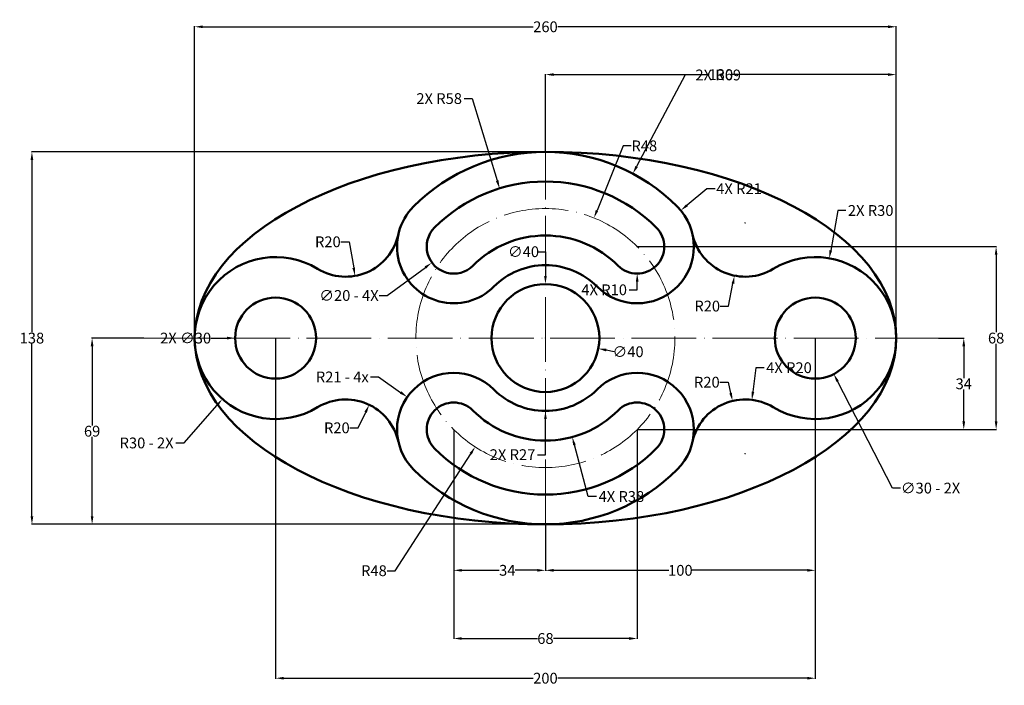
# Model space of a CAD drawing. Units: inches. Extents: x 400 to 765, y 244 to 491.
import ezdxf

# ---------------------------------------------------------------- set-up
doc = ezdxf.new("R2010")
doc.units = ezdxf.units.IN
doc.header["$MEASUREMENT"] = 0
doc.linetypes.add('ACAD_ISO04W100', pattern=[30, 24, -3, 0, -3])
for name, color, linetype, lineweight in [('M-CNTR', 4, 'ACAD_ISO04W100', 18), ('M-CONS', 8, 'Continuous', 13), ('M-DIMS', 7, 'Continuous', 25), ('M-OUTL', 7, 'Continuous', 50)]:
    doc.layers.add(name, color=color, linetype=linetype, lineweight=lineweight)
doc.styles.get("Standard").update_dxf_attribs({"font": 'arial.ttf'})
doc.dimstyles.get("Standard").update_dxf_attribs({"dimtxt": 4, "dimasz": 3, "dimexe": 0.18, "dimexo": 0.0625, "dimgap": 0.09, "dimtad": 0, "dimtih": 1, "dimtoh": 1, "dimdec": 0, "dimzin": 0, "dimdsep": 46, "dimtxsty": 'Standard', "dimcen": 0.09, "dimclrd": 1, "dimclre": 1, "dimadec": 0, "dimazin": 0, "dimtfac": 1, "dimtdec": 0, "dimtofl": 0, "dimtmove": 0, "dimatfit": 3, "dimfxl": 1, "dimtolj": 1, "dimtzin": 0, "dimarcsym": 0})

# ---------------------------------------------------------------- blocks, each defined once
blk = doc.blocks.new('*D1')
at = {"layer": 'Defpoints', "color": 0, "transparency": 16777216}
for p in [(725.07, 488.39), (465.07, 373.06), (725.07, 373.06)]:
    blk.add_point(p, dxfattribs=at)
at = {"layer": 'M-DIMS', "color": 0, "lineweight": -2, "transparency": 16777216}
for p, q in [((465.07, 373.12), (465.07, 488.57)), ((468.07, 488.39), (590.53, 488.39)), ((722.07, 488.39), (599.6, 488.39)), ((725.07, 373.12), (725.07, 488.57))]:
    blk.add_line(p, q, dxfattribs=at)
at = {"layer": 'M-DIMS', "color": 0, "transparency": 16777216}
for points in [[(468.07, 488.89), (468.07, 487.89), (465.07, 488.39)], [(722.07, 488.89), (722.07, 487.89), (725.07, 488.39)]]:
    blk.add_solid(points, dxfattribs=at)
at = {"layer": 'M-DIMS', "color": 0, "transparency": 16777216, "insert": (595.07, 488.39), "char_height": 4, "attachment_point": 5}
blk.add_mtext('\\A1;260', dxfattribs=at)
blk = doc.blocks.new('*D2')
at = {"layer": 'Defpoints', "color": 0, "transparency": 16777216}
for p in [(725.07, 470.68), (595.07, 442.06), (725.07, 373.06)]:
    blk.add_point(p, dxfattribs=at)
at = {"layer": 'M-DIMS', "color": 0, "lineweight": -2, "transparency": 16777216}
for p, q in [((595.07, 442.12), (595.07, 470.86)), ((725.07, 373.12), (725.07, 470.86)), ((598.07, 470.68), (655.75, 470.68)), ((722.07, 470.68), (664.38, 470.68))]:
    blk.add_line(p, q, dxfattribs=at)
at = {"layer": 'M-DIMS', "color": 0, "transparency": 16777216}
for points in [[(598.07, 471.18), (598.07, 470.18), (595.07, 470.68)], [(722.07, 471.18), (722.07, 470.18), (725.07, 470.68)]]:
    blk.add_solid(points, dxfattribs=at)
at = {"layer": 'M-DIMS', "color": 0, "transparency": 16777216, "insert": (660.07, 470.68), "char_height": 4, "attachment_point": 5}
blk.add_mtext('\\A1;130', dxfattribs=at)
blk = doc.blocks.new('*D3')
at = {"layer": 'Defpoints', "color": 0, "transparency": 16777216}
for p in [(595.07, 442.06), (404.77, 304.06), (595.07, 304.06)]:
    blk.add_point(p, dxfattribs=at)
at = {"layer": 'M-DIMS', "color": 0, "lineweight": -2, "transparency": 16777216}
for p, q in [((595.01, 442.06), (404.59, 442.06)), ((404.77, 439.06), (404.77, 375.19)), ((404.77, 307.06), (404.77, 370.93)), ((595.01, 304.06), (404.59, 304.06))]:
    blk.add_line(p, q, dxfattribs=at)
at = {"layer": 'M-DIMS', "color": 0, "transparency": 16777216}
for points in [[(404.27, 439.06), (405.27, 439.06), (404.77, 442.06)], [(404.27, 307.06), (405.27, 307.06), (404.77, 304.06)]]:
    blk.add_solid(points, dxfattribs=at)
at = {"layer": 'M-DIMS', "color": 0, "transparency": 16777216, "insert": (404.77, 373.06), "char_height": 4, "attachment_point": 5}
blk.add_mtext('\\A1;138', dxfattribs=at)
blk = doc.blocks.new('*D4')
at = {"layer": 'Defpoints', "color": 0, "transparency": 16777216}
for p in [(446.33, 373.06), (427.07, 304.06), (595.07, 304.06)]:
    blk.add_point(p, dxfattribs=at)
at = {"layer": 'M-DIMS', "color": 0, "lineweight": -2, "transparency": 16777216}
for p, q in [((446.27, 373.06), (426.89, 373.06)), ((427.07, 370.06), (427.07, 340.69)), ((427.07, 307.06), (427.07, 336.43)), ((595.01, 304.06), (426.89, 304.06))]:
    blk.add_line(p, q, dxfattribs=at)
at = {"layer": 'M-DIMS', "color": 0, "transparency": 16777216}
for points in [[(426.57, 370.06), (427.57, 370.06), (427.07, 373.06)], [(426.57, 307.06), (427.57, 307.06), (427.07, 304.06)]]:
    blk.add_solid(points, dxfattribs=at)
at = {"layer": 'M-DIMS', "color": 0, "transparency": 16777216, "insert": (427.07, 338.56), "char_height": 4, "attachment_point": 5}
blk.add_mtext('\\A1;69', dxfattribs=at)
blk = doc.blocks.new('*D5')
at = {"layer": 'Defpoints', "color": 0, "transparency": 16777216}
for p in [(629.07, 406.94), (629.07, 339.18), (762.09, 339.18)]:
    blk.add_point(p, dxfattribs=at)
at = {"layer": 'M-DIMS', "color": 0, "lineweight": -2, "transparency": 16777216}
for p, q in [((629.13, 406.94), (762.27, 406.94)), ((762.09, 403.94), (762.09, 375.19)), ((762.09, 342.18), (762.09, 370.93)), ((629.13, 339.18), (762.27, 339.18))]:
    blk.add_line(p, q, dxfattribs=at)
at = {"layer": 'M-DIMS', "color": 0, "transparency": 16777216}
for points in [[(761.59, 403.94), (762.59, 403.94), (762.09, 406.94)], [(761.59, 342.18), (762.59, 342.18), (762.09, 339.18)]]:
    blk.add_solid(points, dxfattribs=at)
at = {"layer": 'M-DIMS', "color": 0, "transparency": 16777216, "insert": (762.09, 373.06), "char_height": 4, "attachment_point": 5}
blk.add_mtext('\\A1;68', dxfattribs=at)
blk = doc.blocks.new('*D6')
at = {"layer": 'Defpoints', "color": 0, "transparency": 16777216}
for p in [(740.69, 373.06), (750.1, 373.06), (629.07, 339.18)]:
    blk.add_point(p, dxfattribs=at)
at = {"layer": 'M-DIMS', "color": 0, "lineweight": -2, "transparency": 16777216}
for p, q in [((740.76, 373.06), (750.28, 373.06)), ((750.1, 370.06), (750.1, 358.25)), ((750.1, 342.18), (750.1, 353.99)), ((629.13, 339.18), (750.28, 339.18))]:
    blk.add_line(p, q, dxfattribs=at)
at = {"layer": 'M-DIMS', "color": 0, "transparency": 16777216}
for points in [[(749.6, 370.06), (750.6, 370.06), (750.1, 373.06)], [(749.6, 342.18), (750.6, 342.18), (750.1, 339.18)]]:
    blk.add_solid(points, dxfattribs=at)
at = {"layer": 'M-DIMS', "color": 0, "transparency": 16777216, "insert": (750.1, 356.12), "char_height": 4, "attachment_point": 5}
blk.add_mtext('\\A1;34', dxfattribs=at)
blk = doc.blocks.new('*D7')
at = {"layer": 'Defpoints', "color": 0, "transparency": 16777216}
for p in [(561.07, 339.18), (595.07, 304.06), (595.07, 287.01)]:
    blk.add_point(p, dxfattribs=at)
at = {"layer": 'M-DIMS', "color": 0, "lineweight": -2, "transparency": 16777216}
for p, q in [((561.07, 339.12), (561.07, 286.83)), ((595.07, 304), (595.07, 286.83)), ((564.07, 287.01), (577.98, 287.01)), ((592.07, 287.01), (583.87, 287.01))]:
    blk.add_line(p, q, dxfattribs=at)
at = {"layer": 'M-DIMS', "color": 0, "transparency": 16777216}
for points in [[(564.07, 287.51), (564.07, 286.51), (561.07, 287.01)], [(592.07, 287.51), (592.07, 286.51), (595.07, 287.01)]]:
    blk.add_solid(points, dxfattribs=at)
at = {"layer": 'M-DIMS', "color": 0, "transparency": 16777216, "insert": (580.92, 287.01), "char_height": 4, "attachment_point": 5}
blk.add_mtext('\\A1;34', dxfattribs=at)
blk = doc.blocks.new('*D8')
at = {"layer": 'Defpoints', "color": 0, "transparency": 16777216}
for p in [(561.07, 339.18), (629.07, 339.18), (629.07, 261.75)]:
    blk.add_point(p, dxfattribs=at)
at = {"layer": 'M-DIMS', "color": 0, "lineweight": -2, "transparency": 16777216}
for p, q in [((561.07, 339.12), (561.07, 261.57)), ((629.07, 339.12), (629.07, 261.57)), ((564.07, 261.75), (592.1, 261.75)), ((626.07, 261.75), (598.04, 261.75))]:
    blk.add_line(p, q, dxfattribs=at)
at = {"layer": 'M-DIMS', "color": 0, "transparency": 16777216}
for points in [[(564.07, 262.25), (564.07, 261.25), (561.07, 261.75)], [(626.07, 262.25), (626.07, 261.25), (629.07, 261.75)]]:
    blk.add_solid(points, dxfattribs=at)
at = {"layer": 'M-DIMS', "color": 0, "transparency": 16777216, "insert": (595.07, 261.75), "char_height": 4, "attachment_point": 5}
blk.add_mtext('\\A1;68', dxfattribs=at)
blk = doc.blocks.new('*D9')
at = {"layer": 'Defpoints', "color": 0, "transparency": 16777216}
for p in [(695.07, 373.06), (595.07, 304.06), (695.07, 287.01)]:
    blk.add_point(p, dxfattribs=at)
at = {"layer": 'M-DIMS', "color": 0, "lineweight": -2, "transparency": 16777216}
for p, q in [((695.07, 373), (695.07, 286.83)), ((595.07, 304), (595.07, 286.83)), ((598.07, 287.01), (640.75, 287.01)), ((692.07, 287.01), (649.38, 287.01))]:
    blk.add_line(p, q, dxfattribs=at)
at = {"layer": 'M-DIMS', "color": 0, "transparency": 16777216}
for points in [[(598.07, 287.51), (598.07, 286.51), (595.07, 287.01)], [(692.07, 287.51), (692.07, 286.51), (695.07, 287.01)]]:
    blk.add_solid(points, dxfattribs=at)
at = {"layer": 'M-DIMS', "color": 0, "transparency": 16777216, "insert": (645.07, 287.01), "char_height": 4, "attachment_point": 5}
blk.add_mtext('\\A1;100', dxfattribs=at)
blk = doc.blocks.new('*D10')
at = {"layer": 'Defpoints', "color": 0, "transparency": 16777216}
for p in [(495.07, 373.06), (695.07, 373.06), (695.07, 247.04)]:
    blk.add_point(p, dxfattribs=at)
at = {"layer": 'M-DIMS', "color": 0, "lineweight": -2, "transparency": 16777216}
for p, q in [((495.07, 373), (495.07, 246.86)), ((695.07, 373), (695.07, 246.86)), ((498.07, 247.04), (590.53, 247.04)), ((692.07, 247.04), (599.6, 247.04))]:
    blk.add_line(p, q, dxfattribs=at)
at = {"layer": 'M-DIMS', "color": 0, "transparency": 16777216}
for points in [[(498.07, 247.54), (498.07, 246.54), (495.07, 247.04)], [(692.07, 247.54), (692.07, 246.54), (695.07, 247.04)]]:
    blk.add_solid(points, dxfattribs=at)
at = {"layer": 'M-DIMS', "color": 0, "transparency": 16777216, "insert": (595.07, 247.04), "char_height": 4, "attachment_point": 5}
blk.add_mtext('\\A1;200', dxfattribs=at)
blk = doc.blocks.new('*D11')
at = {"layer": 'Defpoints', "color": 0, "transparency": 16777216}
for p in [(495.07, 373.06), (475.34, 350.46)]:
    blk.add_point(p, dxfattribs=at)
at = {"layer": 'M-DIMS', "color": 0, "lineweight": -2, "transparency": 16777216}
for p, q in [((494.98, 373.06), (495.16, 373.06)), ((495.07, 372.97), (495.07, 373.15)), ((461.14, 334.2), (473.37, 348.2)), ((458.14, 334.2), (461.14, 334.2))]:
    blk.add_line(p, q, dxfattribs=at)
at = {"layer": 'M-DIMS', "color": 0, "transparency": 16777216}
blk.add_solid([(472.99, 348.53), (473.74, 347.87), (475.34, 350.46)], dxfattribs=at)
at = {"layer": 'M-DIMS', "color": 0, "transparency": 16777216, "insert": (447.27, 334.2), "char_height": 4, "attachment_point": 5}
blk.add_mtext('\\A1;R30 - 2X', dxfattribs=at)
blk = doc.blocks.new('*D12')
at = {"layer": 'Defpoints', "color": 0, "transparency": 16777216}
for p in [(529.76, 348.33), (521.03, 330.33)]:
    blk.add_point(p, dxfattribs=at)
at = {"layer": 'M-DIMS', "color": 0, "lineweight": -2, "transparency": 16777216}
for p, q in [((525.63, 339.81), (528.45, 345.63)), ((522.63, 339.81), (525.63, 339.81))]:
    blk.add_line(p, q, dxfattribs=at)
at = {"layer": 'M-DIMS', "color": 0, "transparency": 16777216}
blk.add_solid([(528, 345.84), (528.9, 345.41), (529.76, 348.33)], dxfattribs=at)
at = {"layer": 'M-DIMS', "color": 0, "transparency": 16777216, "insert": (517.77, 339.81), "char_height": 4, "attachment_point": 5}
blk.add_mtext('\\A1;R20', dxfattribs=at)
blk = doc.blocks.new('*D13')
at = {"layer": 'Defpoints', "color": 0, "transparency": 16777216}
for p in [(543.85, 351.2), (561.07, 339.18)]:
    blk.add_point(p, dxfattribs=at)
at = {"layer": 'M-DIMS', "color": 0, "lineweight": -2, "transparency": 16777216}
for p, q in [((530.19, 358.66), (533.19, 358.66)), ((533.19, 358.66), (541.39, 352.92)), ((560.98, 339.18), (561.16, 339.18)), ((561.07, 339.09), (561.07, 339.27))]:
    blk.add_line(p, q, dxfattribs=at)
at = {"layer": 'M-DIMS', "color": 0, "transparency": 16777216}
blk.add_solid([(541.68, 353.33), (541.11, 352.51), (543.85, 351.2)], dxfattribs=at)
at = {"layer": 'M-DIMS', "color": 0, "transparency": 16777216, "insert": (519.78, 358.66), "char_height": 4, "attachment_point": 5}
blk.add_mtext('\\A1;R21 - 4x', dxfattribs=at)
blk = doc.blocks.new('*D14')
at = {"layer": 'Defpoints', "color": 0, "transparency": 16777216}
for p in [(569.13, 412.86), (553.01, 401.02)]:
    blk.add_point(p, dxfattribs=at)
at = {"layer": 'M-DIMS', "color": 0, "lineweight": -2, "transparency": 16777216}
for p, q in [((560.98, 406.94), (561.16, 406.94)), ((561.07, 406.85), (561.07, 407.03)), ((536.4, 388.83), (550.59, 399.25)), ((533.4, 388.83), (536.4, 388.83))]:
    blk.add_line(p, q, dxfattribs=at)
at = {"layer": 'M-DIMS', "color": 0, "transparency": 16777216}
blk.add_solid([(550.29, 399.65), (550.89, 398.85), (553.01, 401.02)], dxfattribs=at)
at = {"layer": 'M-DIMS', "color": 0, "transparency": 16777216, "insert": (522.26, 388.83), "char_height": 4, "attachment_point": 5}
blk.add_mtext('\\A1;∅20 - 4X', dxfattribs=at)
blk = doc.blocks.new('*D15')
at = {"layer": 'Defpoints', "color": 0, "transparency": 16777216}
for p in [(521.03, 415.79), (524.53, 396.1)]:
    blk.add_point(p, dxfattribs=at)
at = {"layer": 'M-DIMS', "color": 0, "lineweight": -2, "transparency": 16777216}
for p, q in [((519.29, 408.73), (522.29, 408.73)), ((522.29, 408.73), (524.01, 399.05))]:
    blk.add_line(p, q, dxfattribs=at)
at = {"layer": 'M-DIMS', "color": 0, "transparency": 16777216}
blk.add_solid([(524.5, 399.14), (523.52, 398.96), (524.53, 396.1)], dxfattribs=at)
at = {"layer": 'M-DIMS', "color": 0, "transparency": 16777216, "insert": (514.43, 408.73), "char_height": 4, "attachment_point": 5}
blk.add_mtext('\\A1;R20', dxfattribs=at)
blk = doc.blocks.new('*D16')
at = {"layer": 'Defpoints', "color": 0, "transparency": 16777216}
for p in [(575.45, 376.96), (614.69, 369.16)]:
    blk.add_point(p, dxfattribs=at)
at = {"layer": 'M-DIMS', "color": 0, "lineweight": -2, "transparency": 16777216}
for p, q in [((594.98, 373.06), (595.16, 373.06)), ((595.07, 372.97), (595.07, 373.15)), ((620.57, 367.99), (617.63, 368.58))]:
    blk.add_line(p, q, dxfattribs=at)
at = {"layer": 'M-DIMS', "color": 0, "transparency": 16777216}
blk.add_solid([(617.73, 369.07), (617.53, 368.09), (614.69, 369.16)], dxfattribs=at)
at = {"layer": 'M-DIMS', "color": 0, "transparency": 16777216, "insert": (625.69, 367.99), "char_height": 4, "attachment_point": 5}
blk.add_mtext('\\A1;∅40', dxfattribs=at)
blk = doc.blocks.new('*D17')
at = {"layer": 'Defpoints', "color": 0, "transparency": 16777216}
for p in [(664.41, 349.77), (669.1, 330.33)]:
    blk.add_point(p, dxfattribs=at)
at = {"layer": 'M-DIMS', "color": 0, "lineweight": -2, "transparency": 16777216}
for p, q in [((659.74, 356.71), (662.74, 356.71)), ((662.74, 356.71), (663.71, 352.69)), ((669.01, 330.33), (669.19, 330.33)), ((669.1, 330.24), (669.1, 330.42))]:
    blk.add_line(p, q, dxfattribs=at)
at = {"layer": 'M-DIMS', "color": 0, "transparency": 16777216}
blk.add_solid([(664.19, 352.81), (663.22, 352.57), (664.41, 349.77)], dxfattribs=at)
at = {"layer": 'M-DIMS', "color": 0, "transparency": 16777216, "insert": (654.88, 356.71), "char_height": 4, "attachment_point": 5}
blk.add_mtext('\\A1;R20', dxfattribs=at)
blk = doc.blocks.new('*D18')
at = {"layer": 'Defpoints', "color": 0, "transparency": 16777216}
for p in [(669.1, 415.79), (665.15, 396.18)]:
    blk.add_point(p, dxfattribs=at)
at = {"layer": 'M-DIMS', "color": 0, "lineweight": -2, "transparency": 16777216}
for p, q in [((669.01, 415.79), (669.19, 415.79)), ((669.1, 415.7), (669.1, 415.88)), ((662.88, 384.92), (664.56, 393.24)), ((659.88, 384.92), (662.88, 384.92))]:
    blk.add_line(p, q, dxfattribs=at)
at = {"layer": 'M-DIMS', "color": 0, "transparency": 16777216}
blk.add_solid([(664.07, 393.34), (665.05, 393.14), (665.15, 396.18)], dxfattribs=at)
at = {"layer": 'M-DIMS', "color": 0, "transparency": 16777216, "insert": (655.02, 384.92), "char_height": 4, "attachment_point": 5}
blk.add_mtext('\\A1;R20', dxfattribs=at)
blk = doc.blocks.new('*D19')
at = {"layer": 'Defpoints', "color": 0, "transparency": 16777216}
for p in [(688.21, 386.4), (701.93, 359.72)]:
    blk.add_point(p, dxfattribs=at)
at = {"layer": 'M-DIMS', "color": 0, "lineweight": -2, "transparency": 16777216}
for p, q in [((694.98, 373.06), (695.16, 373.06)), ((695.07, 372.97), (695.07, 373.15)), ((723.65, 317.48), (703.3, 357.05)), ((726.65, 317.48), (723.65, 317.48))]:
    blk.add_line(p, q, dxfattribs=at)
at = {"layer": 'M-DIMS', "color": 0, "transparency": 16777216}
blk.add_solid([(703.75, 357.28), (702.86, 356.82), (701.93, 359.72)], dxfattribs=at)
at = {"layer": 'M-DIMS', "color": 0, "transparency": 16777216, "insert": (737.79, 317.48), "char_height": 4, "attachment_point": 5}
blk.add_mtext('\\A1;∅30 - 2X', dxfattribs=at)
blk = doc.blocks.new('*D20')
at = {"layer": 'Defpoints', "color": 0, "transparency": 16777216}
for p in [(595.07, 373.06), (569.02, 332.74)]:
    blk.add_point(p, dxfattribs=at)
at = {"layer": 'M-DIMS', "color": 0, "lineweight": -2, "transparency": 16777216}
for p, q in [((594.98, 373.06), (595.16, 373.06)), ((595.07, 372.97), (595.07, 373.15)), ((539.38, 286.87), (567.39, 330.22)), ((536.38, 286.87), (539.38, 286.87))]:
    blk.add_line(p, q, dxfattribs=at)
at = {"layer": 'M-DIMS', "color": 0, "transparency": 16777216}
blk.add_solid([(566.97, 330.49), (567.81, 329.95), (569.02, 332.74)], dxfattribs=at)
at = {"layer": 'M-DIMS', "color": 0, "transparency": 16777216, "insert": (531.51, 286.87), "char_height": 4, "attachment_point": 5}
blk.add_mtext('\\A1;R48', dxfattribs=at)
blk = doc.blocks.new('LINK-CURVED-SLOT')
for centre, radius, start, end in [((-34, -33.88), 21, 44.9005, 224.9005), ((34, -33.88), 21, 315.0995, 135.0995), ((0, 0), 27, 224.9005, 315.0995), ((-34, -33.88), 10, 44.9005, 224.9005), ((34, -33.88), 10, 315.0995, 135.0995), ((0, 0), 38, 224.9005, 315.0995), ((0, 0), 58, 224.9005, 315.0995), ((0, 0), 69, 224.9005, 315.0995)]:
    blk.add_arc(centre, radius, start, end)
blk = doc.blocks.new('LINK-MOUNTING-EYE')
blk.add_circle((0, 0), 15)
for centre, radius, start, end in [((25.97, 42.73), 20, 238.7135, 347.5388), ((0, 0), 30, 58.7135, 301.2865), ((25.97, -42.73), 20, 12.4612, 121.2865)]:
    blk.add_arc(centre, radius, start, end)
blk = doc.blocks.new('*D23')
at = {"layer": 'Defpoints', "color": 0, "transparency": 16777216}
for p in [(595.07, 393.06), (595.07, 353.06)]:
    blk.add_point(p, dxfattribs=at)
at = {"layer": 'M-DIMS', "color": 1, "lineweight": -2, "transparency": 16777216}
for p, q in [((592.07, 405.06), (595.07, 405.06)), ((595.07, 405.06), (595.07, 396.06)), ((594.98, 373.06), (595.16, 373.06)), ((595.07, 372.97), (595.07, 373.15))]:
    blk.add_line(p, q, dxfattribs=at)
at = {"layer": 'M-DIMS', "color": 1, "transparency": 16777216}
blk.add_solid([(595.57, 396.06), (594.57, 396.06), (595.07, 393.06)], dxfattribs=at)
at = {"layer": 'M-DIMS', "color": 0, "transparency": 16777216, "insert": (586.94, 405.06), "char_height": 4, "attachment_point": 5}
blk.add_mtext('\\A1;∅40', dxfattribs=at)
blk = doc.blocks.new('*D24')
at = {"layer": 'Defpoints', "color": 0, "transparency": 16777216}
for p in [(480.07, 373.06), (510.07, 373.06)]:
    blk.add_point(p, dxfattribs=at)
at = {"layer": 'M-DIMS', "color": 1, "lineweight": -2, "transparency": 16777216}
for p, q in [((471.07, 373.06), (477.07, 373.06)), ((494.98, 373.06), (495.16, 373.06)), ((495.07, 372.97), (495.07, 373.15))]:
    blk.add_line(p, q, dxfattribs=at)
at = {"layer": 'M-DIMS', "color": 1, "transparency": 16777216}
blk.add_solid([(477.07, 373.56), (477.07, 372.56), (480.07, 373.06)], dxfattribs=at)
at = {"layer": 'M-DIMS', "color": 0, "transparency": 16777216, "insert": (461.72, 373.06), "char_height": 4, "attachment_point": 5}
blk.add_mtext('\\A1;2X ∅30', dxfattribs=at)
blk = doc.blocks.new('*D25')
at = {"layer": 'Defpoints', "color": 0, "transparency": 16777216}
for p in [(671.59, 350.18), (669.1, 330.33)]:
    blk.add_point(p, dxfattribs=at)
at = {"layer": 'M-DIMS', "color": 1, "lineweight": -2, "transparency": 16777216}
for p, q in [((673.08, 362.08), (671.96, 353.15)), ((676.08, 362.08), (673.08, 362.08)), ((669.01, 330.33), (669.19, 330.33)), ((669.1, 330.24), (669.1, 330.42))]:
    blk.add_line(p, q, dxfattribs=at)
at = {"layer": 'M-DIMS', "color": 1, "transparency": 16777216}
blk.add_solid([(671.46, 353.21), (672.46, 353.09), (671.59, 350.18)], dxfattribs=at)
at = {"layer": 'M-DIMS', "color": 0, "transparency": 16777216, "insert": (685.32, 362.08), "char_height": 4, "attachment_point": 5}
blk.add_mtext('\\A1;4X R20', dxfattribs=at)
blk = doc.blocks.new('*D26')
at = {"layer": 'Defpoints', "color": 0, "transparency": 16777216}
for p in [(645.23, 420.35), (629.07, 406.94)]:
    blk.add_point(p, dxfattribs=at)
at = {"layer": 'M-DIMS', "color": 1, "lineweight": -2, "transparency": 16777216}
for p, q in [((654.93, 428.39), (647.54, 422.26)), ((657.93, 428.39), (654.93, 428.39)), ((628.98, 406.94), (629.16, 406.94)), ((629.07, 406.85), (629.07, 407.03))]:
    blk.add_line(p, q, dxfattribs=at)
at = {"layer": 'M-DIMS', "color": 1, "transparency": 16777216}
blk.add_solid([(647.22, 422.65), (647.86, 421.88), (645.23, 420.35)], dxfattribs=at)
at = {"layer": 'M-DIMS', "color": 0, "transparency": 16777216, "insert": (666.8, 428.39), "char_height": 4, "attachment_point": 5}
blk.add_mtext('\\A1;4X R21', dxfattribs=at)
blk = doc.blocks.new('*D27')
at = {"layer": 'Defpoints', "color": 0, "transparency": 16777216}
for p in [(629.07, 406.94), (629.07, 396.94)]:
    blk.add_point(p, dxfattribs=at)
at = {"layer": 'M-DIMS', "color": 1, "lineweight": -2, "transparency": 16777216}
for p, q in [((628.98, 406.94), (629.16, 406.94)), ((629.07, 406.85), (629.07, 407.03)), ((626.07, 390.94), (629.07, 390.94)), ((629.07, 390.94), (629.07, 393.94))]:
    blk.add_line(p, q, dxfattribs=at)
at = {"layer": 'M-DIMS', "color": 1, "transparency": 16777216}
blk.add_solid([(628.57, 393.94), (629.57, 393.94), (629.07, 396.94)], dxfattribs=at)
at = {"layer": 'M-DIMS', "color": 0, "transparency": 16777216, "insert": (616.83, 390.94), "char_height": 4, "attachment_point": 5}
blk.add_mtext('\\A1;4X R10', dxfattribs=at)
blk = doc.blocks.new('*D28')
at = {"layer": 'Defpoints', "color": 0, "transparency": 16777216}
for p in [(700.28, 402.6), (695.07, 373.06)]:
    blk.add_point(p, dxfattribs=at)
at = {"layer": 'M-DIMS', "color": 1, "lineweight": -2, "transparency": 16777216}
for p, q in [((703.41, 420.33), (700.8, 405.56)), ((706.41, 420.33), (703.41, 420.33)), ((694.98, 373.06), (695.16, 373.06)), ((695.07, 372.97), (695.07, 373.15))]:
    blk.add_line(p, q, dxfattribs=at)
at = {"layer": 'M-DIMS', "color": 1, "transparency": 16777216}
blk.add_solid([(700.31, 405.65), (701.29, 405.47), (700.28, 402.6)], dxfattribs=at)
at = {"layer": 'M-DIMS', "color": 0, "transparency": 16777216, "insert": (715.6, 420.33), "char_height": 4, "attachment_point": 5}
blk.add_mtext('\\A1;2X R30', dxfattribs=at)
blk = doc.blocks.new('*D29')
at = {"layer": 'Defpoints', "color": 0, "transparency": 16777216}
for p in [(627.46, 433.99), (595.07, 373.06)]:
    blk.add_point(p, dxfattribs=at)
at = {"layer": 'M-DIMS', "color": 1, "lineweight": -2, "transparency": 16777216}
for p, q in [((646.89, 470.54), (628.87, 436.63)), ((649.89, 470.54), (646.89, 470.54)), ((594.98, 373.06), (595.16, 373.06)), ((595.07, 372.97), (595.07, 373.15))]:
    blk.add_line(p, q, dxfattribs=at)
at = {"layer": 'M-DIMS', "color": 1, "transparency": 16777216}
blk.add_solid([(628.42, 436.87), (629.31, 436.4), (627.46, 433.99)], dxfattribs=at)
at = {"layer": 'M-DIMS', "color": 0, "transparency": 16777216, "insert": (659.1, 470.54), "char_height": 4, "attachment_point": 5}
blk.add_mtext('\\A1;2X R69', dxfattribs=at)
blk = doc.blocks.new('*D30')
at = {"layer": 'Defpoints', "color": 0, "transparency": 16777216}
for p in [(578.08, 428.52), (595.07, 373.06)]:
    blk.add_point(p, dxfattribs=at)
at = {"layer": 'M-DIMS', "color": 1, "lineweight": -2, "transparency": 16777216}
for p, q in [((564.89, 461.79), (567.89, 461.79)), ((567.89, 461.79), (577.2, 431.39)), ((594.98, 373.06), (595.16, 373.06)), ((595.07, 372.97), (595.07, 373.15))]:
    blk.add_line(p, q, dxfattribs=at)
at = {"layer": 'M-DIMS', "color": 1, "transparency": 16777216}
blk.add_solid([(577.68, 431.53), (576.72, 431.24), (578.08, 428.52)], dxfattribs=at)
at = {"layer": 'M-DIMS', "color": 0, "transparency": 16777216, "insert": (555.68, 461.79), "char_height": 4, "attachment_point": 5}
blk.add_mtext('\\A1;2X R58', dxfattribs=at)
blk = doc.blocks.new('*D31')
at = {"layer": 'Defpoints', "color": 0, "transparency": 16777216}
for p in [(595.07, 373.06), (605, 336.38)]:
    blk.add_point(p, dxfattribs=at)
at = {"layer": 'M-DIMS', "color": 1, "lineweight": -2, "transparency": 16777216}
for p, q in [((594.98, 373.06), (595.16, 373.06)), ((595.07, 372.97), (595.07, 373.15)), ((610.96, 314.37), (605.78, 333.49)), ((613.96, 314.37), (610.96, 314.37))]:
    blk.add_line(p, q, dxfattribs=at)
at = {"layer": 'M-DIMS', "color": 1, "transparency": 16777216}
blk.add_solid([(606.27, 333.62), (605.3, 333.35), (605, 336.38)], dxfattribs=at)
at = {"layer": 'M-DIMS', "color": 0, "transparency": 16777216, "insert": (623.21, 314.37), "char_height": 4, "attachment_point": 5}
blk.add_mtext('\\A1;4X R38', dxfattribs=at)
blk = doc.blocks.new('*D32')
at = {"layer": 'Defpoints', "color": 0, "transparency": 16777216}
for p in [(595.07, 373.06), (595.07, 346.06)]:
    blk.add_point(p, dxfattribs=at)
at = {"layer": 'M-DIMS', "color": 1, "lineweight": -2, "transparency": 16777216}
for p, q in [((594.98, 373.06), (595.16, 373.06)), ((595.07, 372.97), (595.07, 373.15)), ((595.07, 329.86), (595.07, 343.06)), ((592.07, 329.86), (595.07, 329.86))]:
    blk.add_line(p, q, dxfattribs=at)
at = {"layer": 'M-DIMS', "color": 1, "transparency": 16777216}
blk.add_solid([(594.57, 343.06), (595.57, 343.06), (595.07, 346.06)], dxfattribs=at)
at = {"layer": 'M-DIMS', "color": 0, "transparency": 16777216, "insert": (582.87, 329.86), "char_height": 4, "attachment_point": 5}
blk.add_mtext('\\A1;2X R27', dxfattribs=at)
blk = doc.blocks.new('*D33')
at = {"layer": 'Defpoints', "color": 0, "transparency": 16777216}
for p in [(613.05, 417.56), (595.07, 373.06)]:
    blk.add_point(p, dxfattribs=at)
at = {"layer": 'M-DIMS', "color": 1, "lineweight": -2, "transparency": 16777216}
for p, q in [((623.84, 444.27), (614.18, 420.35)), ((626.84, 444.27), (623.84, 444.27)), ((594.98, 373.06), (595.16, 373.06)), ((595.07, 372.97), (595.07, 373.15))]:
    blk.add_line(p, q, dxfattribs=at)
at = {"layer": 'M-DIMS', "color": 1, "transparency": 16777216}
blk.add_solid([(613.71, 420.53), (614.64, 420.16), (613.05, 417.56)], dxfattribs=at)
at = {"layer": 'M-DIMS', "color": 0, "transparency": 16777216, "insert": (631.71, 444.27), "char_height": 4, "attachment_point": 5}
blk.add_mtext('\\A1;R48', dxfattribs=at)

msp = doc.modelspace()

# ---------------------------------------------------------------- linework, layer by layer
at = {"layer": 'M-CNTR'}
for p, q in [((595.07, 304.06), (595.07, 442.06)), ((446.33, 373.06), (740.69, 373.06))]:
    msp.add_line(p, q, dxfattribs=at)
msp.add_circle((595.07, 373.06), 48, dxfattribs=at)
at = {"layer": 'M-CONS'}
for start, end in [(199.6293, 199.9299), (340.0701, 340.3707)]:
    msp.add_arc((595.07, 373.06), 38, start, end, dxfattribs=at)
at = {"layer": 'M-OUTL'}
msp.add_circle((595.07, 373.06), 20, dxfattribs=at)
msp.add_ellipse((595.07, 373.06), major_axis=(130, 0), ratio=0.530769, dxfattribs=at)

# ---------------------------------------------------------------- block references
at = {"layer": 'M-OUTL', "rotation": 180}
for name, p in [('LINK-CURVED-SLOT', (595.07, 373.06)), ('LINK-MOUNTING-EYE', (695.07, 373.06))]:
    msp.add_blockref(name, p, dxfattribs=at)
at = {"layer": 'M-OUTL'}
for name, p in [('LINK-MOUNTING-EYE', (495.07, 373.06)), ('LINK-CURVED-SLOT', (595.07, 373.06))]:
    msp.add_blockref(name, p, dxfattribs=at)

# ---------------------------------------------------------------- dimensions: what is measured, and where the dimension line sits
at = {"layer": 'M-DIMS'}
for base, p1, p2, picture, middle in [((725.07, 488.39), (465.07, 373.06), (725.07, 373.06), '*D1', (595.07, 488.39)), ((725.07, 470.68), (595.07, 442.06), (725.07, 373.06), '*D2', (660.07, 470.68)), ((695.07, 247.04), (495.07, 373.06), (695.07, 373.06), '*D10', (595.07, 247.04)), ((695.07, 287.01), (595.07, 304.06), (695.07, 373.06), '*D9', (645.07, 287.01))]:
    dim = msp.add_linear_dim(base=base, p1=p1, p2=p2, dimstyle='Standard', override={"dimclrd": 0, "dimclre": 0, "dimclrt": 0}, dxfattribs=at)
    dim.commit()
    dim.dimension.update_dxf_attribs({"geometry": picture, "text_midpoint": middle})
for center, mpoint, text, override, picture, middle in [((595.07, 373.06), (627.46, 433.99), '2X <>', {"dimdec": 0, "dimlfac": 1, "dimrnd": 0, "dimzin": 0, "dimdsep": 46, "dimlunit": 2}, '*D29', (659.1, 470.54)), ((595.07, 373.06), (578.08, 428.52), '2X <>', {"dimdec": 0, "dimlfac": 1, "dimrnd": 0, "dimzin": 0, "dimdsep": 46, "dimlunit": 2}, '*D30', (555.68, 461.79)), ((629.07, 406.94), (645.23, 420.35), '4X <>', {"dimdec": 0, "dimlfac": 1, "dimrnd": 0, "dimzin": 0, "dimdsep": 46, "dimlunit": 2}, '*D26', (666.8, 428.39)), ((695.07, 373.06), (700.28, 402.6), '2X <>', {"dimdec": 0, "dimlfac": 1, "dimrnd": 0, "dimzin": 0, "dimdsep": 46, "dimlunit": 2}, '*D28', (715.6, 420.33)), ((629.07, 406.94), (629.07, 396.94), '4X <>', {"dimdec": 0, "dimlfac": 1, "dimrnd": 0, "dimzin": 0, "dimdsep": 46, "dimlunit": 2}, '*D27', (616.83, 390.94)), ((495.07, 373.06), (475.34, 350.46), '<> - 2X', {"dimclrd": 0, "dimclre": 0, "dimclrt": 0}, '*D11', (447.27, 334.2)), ((595.07, 373.06), (595.07, 346.06), '2X <>', {"dimdec": 0, "dimlfac": 1, "dimrnd": 0, "dimzin": 0, "dimdsep": 46, "dimlunit": 2}, '*D32', (582.87, 329.86)), ((595.07, 373.06), (605, 336.38), '4X <>', {"dimdec": 0, "dimlfac": 1, "dimrnd": 0, "dimzin": 0, "dimdsep": 46, "dimlunit": 2}, '*D31', (623.21, 314.37)), ((561.07, 339.18), (543.85, 351.2), '<> - 4x', {"dimclrd": 0, "dimclre": 0, "dimclrt": 0}, '*D13', (519.78, 358.66)), ((669.1, 330.33), (671.59, 350.18), '4X <>', {"dimdec": 0, "dimlfac": 1, "dimrnd": 0, "dimzin": 0, "dimdsep": 46, "dimlunit": 2}, '*D25', (685.32, 362.08))]:
    dim = msp.add_radius_dim(center=center, mpoint=mpoint, text=text, dimstyle='Standard', override=override, dxfattribs=at)
    dim.commit()
    dim.dimension.update_dxf_attribs({"geometry": picture, "text_midpoint": middle, "dimtype": 164})
for center, mpoint, override, picture, middle in [((595.07, 373.06), (613.05, 417.56), {"dimdec": 0, "dimlfac": 1, "dimrnd": 0, "dimzin": 0, "dimdsep": 46, "dimlunit": 2}, '*D33', (631.71, 444.27)), ((521.03, 415.79), (524.53, 396.1), {"dimclrd": 0, "dimclre": 0, "dimclrt": 0}, '*D15', (514.43, 408.73)), ((669.1, 415.79), (665.15, 396.18), {"dimclrd": 0, "dimclre": 0, "dimclrt": 0}, '*D18', (655.02, 384.92)), ((595.07, 373.06), (569.02, 332.74), {"dimclrd": 0, "dimclre": 0, "dimclrt": 0}, '*D20', (531.51, 286.87)), ((669.1, 330.33), (664.41, 349.77), {"dimclrd": 0, "dimclre": 0, "dimclrt": 0}, '*D17', (654.88, 356.71)), ((521.03, 330.33), (529.76, 348.33), {"dimclrd": 0, "dimclre": 0, "dimclrt": 0}, '*D12', (517.77, 339.81))]:
    dim = msp.add_radius_dim(center=center, mpoint=mpoint, dimstyle='Standard', override=override, dxfattribs=at)
    dim.commit()
    dim.dimension.update_dxf_attribs({"geometry": picture, "text_midpoint": middle, "dimtype": 164})
for base, p1, p2, picture, middle in [((404.77, 304.06), (595.07, 442.06), (595.07, 304.06), '*D3', (404.77, 373.06)), ((762.09, 339.18), (629.07, 406.94), (629.07, 339.18), '*D5', (762.09, 373.06)), ((427.07, 304.06), (446.33, 373.06), (595.07, 304.06), '*D4', (427.07, 338.56)), ((750.1, 373.06), (629.07, 339.18), (740.69, 373.06), '*D6', (750.1, 356.12))]:
    dim = msp.add_linear_dim(base=base, p1=p1, p2=p2, angle=90, dimstyle='Standard', override={"dimclrd": 0, "dimclre": 0, "dimclrt": 0}, dxfattribs=at)
    dim.commit()
    dim.dimension.update_dxf_attribs({"geometry": picture, "text_midpoint": middle})
for p1, p2, text, override, picture, middle in [((569.13, 412.86), (553.01, 401.02), '<> - 4X', {"dimclrd": 0, "dimclre": 0, "dimclrt": 0}, '*D14', (522.26, 388.83)), ((688.21, 386.4), (701.93, 359.72), '<> - 2X', {"dimclrd": 0, "dimclre": 0, "dimclrt": 0}, '*D19', (737.79, 317.48)), ((510.07, 373.06), (480.07, 373.06), '2X <>', {"dimdec": 0, "dimlfac": 1, "dimrnd": 0, "dimzin": 0, "dimdsep": 46, "dimlunit": 2}, '*D24', (471.07, 373.06))]:
    dim = msp.add_diameter_dim_2p(p1=p1, p2=p2, text=text, dimstyle='Standard', override=override, dxfattribs=at)
    dim.commit()
    dim.dimension.update_dxf_attribs({"geometry": picture, "text_midpoint": middle, "dimtype": 163})
for p1, p2, override, picture, middle in [((595.07, 353.06), (595.07, 393.06), {"dimdec": 0, "dimlfac": 1, "dimrnd": 0, "dimzin": 0, "dimdsep": 46, "dimlunit": 2}, '*D23', (586.94, 405.06)), ((575.45, 376.96), (614.69, 369.16), {"dimclrd": 0, "dimclre": 0, "dimclrt": 0}, '*D16', (620.57, 367.99))]:
    dim = msp.add_diameter_dim_2p(p1=p1, p2=p2, dimstyle='Standard', override=override, dxfattribs=at)
    dim.commit()
    dim.dimension.update_dxf_attribs({"geometry": picture, "text_midpoint": middle, "dimtype": 163})
for base, p2, picture, middle in [((595.07, 287.01), (595.07, 304.06), '*D7', (580.92, 287.01)), ((629.07, 261.75), (629.07, 339.18), '*D8', (595.07, 261.75))]:
    dim = msp.add_linear_dim(base=base, p1=(561.07, 339.18), p2=p2, dimstyle='Standard', override={"dimclrd": 0, "dimclre": 0, "dimclrt": 0}, dxfattribs=at)
    dim.commit()
    dim.dimension.update_dxf_attribs({"geometry": picture, "text_midpoint": middle, "dimtype": 160})

doc.saveas('drawing.dxf')
